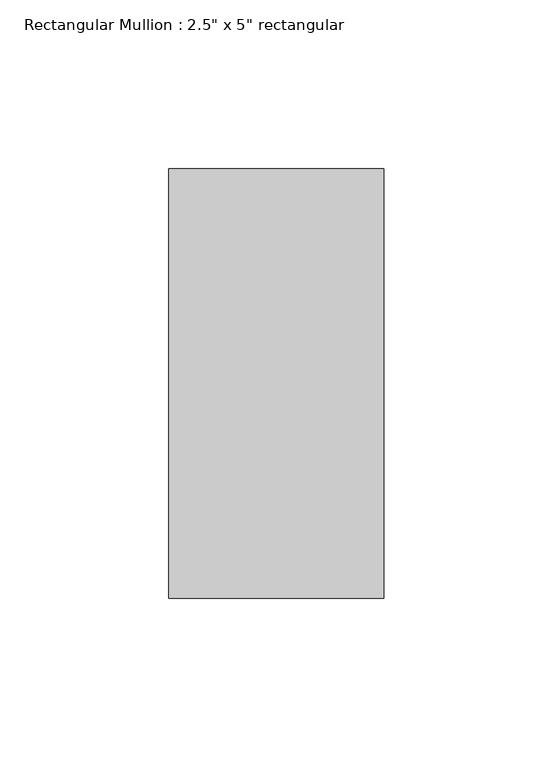
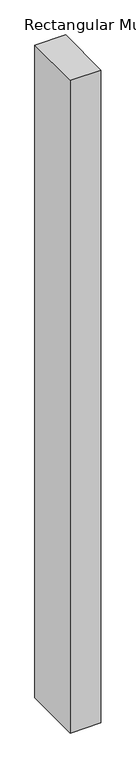
"""IFC4 building model written with IfcOpenShell, lengths in millimetres: member geometry."""

from ifc_helpers import new_model, si_unit, frame, origin, place, context, project, spatial, polyline, outline, extrude, source, transform, mapped, element, save


def member_3ae3f724(model_context):
    return source(origin(), model_context, "Body", "SweptSolid", [
        extrude(outline(polyline([(31.75, 63.5), (31.75, -63.5), (-31.75, -63.5), (-31.75, 63.5), (31.75, 63.5)])), frame((0.0, 0.0, -1431.1740318), z_axis=(0.0, 0.0, 1.0), x_axis=(1.0, 0.0, 0.0)), (0.0, 0.0, 1.0), 1431.1740318),
    ])


if __name__ == "__main__":
    model = new_model("IFC4")
    model_context = context("Model", 3, world=origin())
    ifc_project = project(units=[si_unit("LENGTHUNIT", "METRE", prefix="MILLI")], contexts=[model_context])
    site = spatial("IfcSite", under=ifc_project)
    building = spatial("IfcBuilding", under=site)
    placement = place(None, origin())
    member_shape = member_3ae3f724(model_context)
    element("IfcMember", 1, ObjectType="Rectangular Mullion : 2.5\" x 5\" rectangular", at=placement, inside=building, context=model_context, shape_type="MappedRepresentation", body=[
        mapped(member_shape, transform((0.0, 0.0, 0.0), x_axis=(1.0, 0.0, 0.0), y_axis=(0.0, 1.0, 0.0), z_axis=(0.0, 0.0, 1.0))),
    ])
    save(model, "model.ifc")

# Revit data of these elements
# Type "Rectangular Mullion : 2.5\" x 5\" rectangular"
#   built-in parameter 1007304 = 0.416667 (stored number, unit not read)
#   built-in parameter 1007301 = 0.104167 (stored number, unit not read)
#   built-in parameter 1007300 = 0.104167 (stored number, unit not read)
# Element 1 (IfcMember, "Rectangular Mullion : 2.5\" x 5\" rectangular")
#   Materials on its faces: "Aluminum"
# Materials
#   "Aluminum": class "Metal", colour RGB 247 247 247, transparency 0, Description = "Aluminum 6061", Cost = 0
